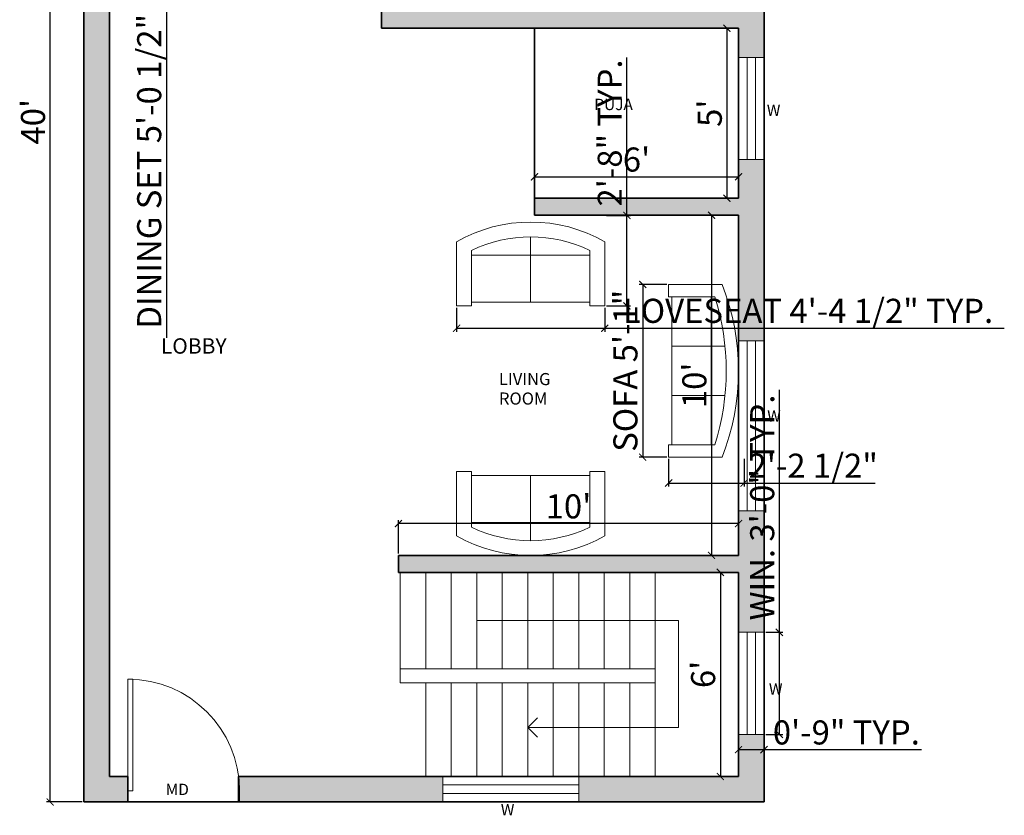
# Model space of a CAD drawing. Units: inches. Extents: x 3799 to 20199, y 1682 to 8087.
# Tile 28 of 30: x 17373 to 17720, y 7238 to 7519. Entities that reach past the tile are written whole.
import ezdxf

# ---------------------------------------------------------------- set-up
doc = ezdxf.new("R2010")
doc.units = ezdxf.units.IN
for name, color, linetype, lineweight in [('A-ANNO-DIMS', 2, 'Continuous', 18), ('A-ANNO-SYMB', 3, 'Continuous', 18), ('A-AREA-IDEN', 7, 'Continuous', 18), ('A-DOOR', 3, 'Continuous', 18), ('A-FLOR-STRS', 41, 'Continuous', 18), ('A-FURN', 8, 'Continuous', 18), ('A-GLAZ', 152, 'Continuous', 18), ('A-WALL', 7, 'Continuous', 35), ('A-WALL-PATT', 252, 'Continuous', 13)]:
    doc.layers.add(name, color=color, linetype=linetype, lineweight=lineweight)
doc.styles.get("Standard").update_dxf_attribs({"font": 'arial.ttf'})
doc.dimstyles.new('ISO-25', dxfattribs={"dimtxt": 8.5, "dimasz": 2.5, "dimexe": 1.25, "dimexo": 0.625, "dimtad": 1, "dimdec": 0, "dimlunit": 3, "dimtxsty": 'Standard', "dimblk": 'ARCHTICK', "dimcen": 2.5, "dimadec": 0, "dimazin": 0, "dimtfac": 1, "dimtdec": 0, "dimtmove": 0, "dimatfit": 3, "dimfxl": 1, "dimarcsym": 0})

# ---------------------------------------------------------------- blocks, each defined once
blk = doc.blocks.new('*U158')
for p, q in [((0, 0), (0, -100)), ((1000, 0), (1000, -100))]:
    blk.add_line(p, q)
blk.add_lwpolyline([(0, 0), (0, 1000), (43.75, 1000), (43.75, 0)], close=True)
blk.add_arc((0, 0), 1000, 0, 90)
blk = doc.blocks.new('Sofa - Roundback Loveseat 5 ft.')
for p, q in [((0, -32.44198), (0, -5.99998)), ((-24, -33.99998), (-24, -11.46958)), ((24.00004, -33.99998), (24.00004, -11.46958)), ((-23.9998, -13.38178), (23.99986, -13.38178)), ((-24, -32.44198), (24.00004, -32.44198))]:
    blk.add_line(p, q)
for points in [[(-24, -33.99998), (-30, -33.99998), (-30, -7.99998)], [(30.00004, -7.99998), (30.00004, -33.99998), (24.00004, -33.99998)]]:
    blk.add_lwpolyline(points)
for centre, radius, start, end in [((0, -60.24998), 60.24998, 60.13715, 119.8628), ((0, -61.38438), 55.38444, 64.32083, 115.6792)]:
    blk.add_arc(centre, radius, start, end)
blk = doc.blocks.new('Sofa - Roundback 7 ft.')
for p, q in [((-12.00002, -32.4421), (-12.00003, -6.5971)), ((11.99997, -32.4421), (11.99998, -6.5971)), ((-36.000027, -34), (-36.000027, -11.4696)), ((-35.999844, -13.3819), (35.9998, -13.3819)), ((35.99998, -34), (35.99998, -11.4696)), ((-36.000027, -32.4421), (35.99998, -32.4421))]:
    blk.add_line(p, q)
for points in [[(-36.000027, -34), (-42.000027, -34), (-42.000027, -8)], [(41.99998, -8), (41.99998, -34), (35.99998, -34)]]:
    blk.add_lwpolyline(points)
for centre, radius, start, end in [((0, -114.25), 114.25, 68.43141, 111.5686), ((-0.00001, -127.1968), 121.1968, 72.72033, 107.2797)]:
    blk.add_arc(centre, radius, start, end)
blk = doc.blocks.new('_ArchTick')
at = {"color": 0, "linetype": 'ByBlock', "const_width": 0.15}
blk.add_lwpolyline([(-0.5, -0.5), (0.5, 0.5)], dxfattribs=at)
blk = doc.blocks.new('*D163')
at = {"layer": 'A-ANNO-DIMS', "color": 0, "lineweight": -2, "transparency": 16777216}
for p, q in [((17554.17, 7456.64), (17554.17, 7464.85)), ((17554.17, 7463.6), (17626.17, 7463.6)), ((17626.17, 7456.64), (17626.17, 7464.85))]:
    blk.add_line(p, q, dxfattribs=at)
at = {"layer": 'Defpoints', "color": 0, "transparency": 16777216}
for p in [(17626.17, 7463.6), (17554.17, 7456.02), (17626.17, 7456.02)]:
    blk.add_point(p, dxfattribs=at)
at = {"layer": 'A-ANNO-DIMS', "color": 0, "lineweight": -2, "transparency": 16777216, "xscale": 2.5, "yscale": 2.5, "zscale": 2.5, "rotation": 180}
blk.add_blockref('_ArchTick', (17554.17, 7463.6), dxfattribs=at)
at = {"layer": 'A-ANNO-DIMS', "color": 0, "lineweight": -2, "transparency": 16777216, "xscale": 2.5, "yscale": 2.5, "zscale": 2.5}
blk.add_blockref('_ArchTick', (17626.17, 7463.6), dxfattribs=at)
at = {"layer": 'A-ANNO-DIMS', "color": 0, "transparency": 16777216, "insert": (17590.17, 7468.57), "char_height": 8.5, "attachment_point": 5}
blk.add_mtext("6'", dxfattribs=at)
blk = doc.blocks.new('*D164')
at = {"layer": 'A-ANNO-DIMS', "color": 0, "lineweight": -2, "transparency": 16777216}
for p, q in [((17625.55, 7516.02), (17620.81, 7516.02)), ((17622.06, 7516.02), (17622.06, 7456.02)), ((17625.55, 7456.02), (17620.81, 7456.02))]:
    blk.add_line(p, q, dxfattribs=at)
at = {"layer": 'Defpoints', "color": 0, "transparency": 16777216}
for p in [(17626.17, 7516.02), (17622.06, 7456.02), (17626.17, 7456.02)]:
    blk.add_point(p, dxfattribs=at)
at = {"layer": 'A-ANNO-DIMS', "color": 0, "lineweight": -2, "transparency": 16777216, "xscale": 2.5, "yscale": 2.5, "zscale": 2.5}
for p, rotation in [((17622.06, 7516.02), 90), ((17622.06, 7456.02), 270)]:
    blk.add_blockref('_ArchTick', p, dxfattribs=dict(at, rotation=rotation))
at = {"layer": 'A-ANNO-DIMS', "color": 0, "transparency": 16777216, "insert": (17617.11, 7486.02), "char_height": 8.5, "attachment_point": 5, "rotation": 90}
blk.add_mtext("5'", dxfattribs=at)
blk = doc.blocks.new('*D165')
at = {"layer": 'A-ANNO-DIMS', "color": 0, "lineweight": -2, "transparency": 16777216}
for p, q in [((17625.55, 7324.02), (17618.49, 7324.02)), ((17619.74, 7324.02), (17619.74, 7252.02)), ((17625.55, 7252.02), (17618.49, 7252.02))]:
    blk.add_line(p, q, dxfattribs=at)
at = {"layer": 'Defpoints', "color": 0, "transparency": 16777216}
for p in [(17626.17, 7324.02), (17619.74, 7252.02), (17626.17, 7252.02)]:
    blk.add_point(p, dxfattribs=at)
at = {"layer": 'A-ANNO-DIMS', "color": 0, "lineweight": -2, "transparency": 16777216, "xscale": 2.5, "yscale": 2.5, "zscale": 2.5}
for p, rotation in [((17619.74, 7324.02), 90), ((17619.74, 7252.02), 270)]:
    blk.add_blockref('_ArchTick', p, dxfattribs=dict(at, rotation=rotation))
at = {"layer": 'A-ANNO-DIMS', "color": 0, "transparency": 16777216, "insert": (17614.77, 7288.02), "char_height": 8.5, "attachment_point": 5, "rotation": 90}
blk.add_mtext("6'", dxfattribs=at)
blk = doc.blocks.new('*D166')
at = {"layer": 'A-ANNO-DIMS', "color": 0, "lineweight": -2, "transparency": 16777216}
for p, q in [((17625.55, 7450.02), (17615.39, 7450.02)), ((17616.64, 7450.02), (17616.64, 7330.02)), ((17625.55, 7330.02), (17615.39, 7330.02))]:
    blk.add_line(p, q, dxfattribs=at)
at = {"layer": 'Defpoints', "color": 0, "transparency": 16777216}
for p in [(17626.17, 7450.02), (17616.64, 7330.02), (17626.17, 7330.02)]:
    blk.add_point(p, dxfattribs=at)
at = {"layer": 'A-ANNO-DIMS', "color": 0, "lineweight": -2, "transparency": 16777216, "xscale": 2.5, "yscale": 2.5, "zscale": 2.5}
for p, rotation in [((17616.64, 7450.02), 90), ((17616.64, 7330.02), 270)]:
    blk.add_blockref('_ArchTick', p, dxfattribs=dict(at, rotation=rotation))
at = {"layer": 'A-ANNO-DIMS', "color": 0, "transparency": 16777216, "insert": (17611.68, 7390.02), "char_height": 8.5, "attachment_point": 5, "rotation": 90}
blk.add_mtext("10'", dxfattribs=at)
blk = doc.blocks.new('*D167')
at = {"layer": 'A-ANNO-DIMS', "color": 0, "lineweight": -2, "transparency": 16777216}
for p, q in [((17506.17, 7330.64), (17506.17, 7342.49)), ((17626.17, 7341.24), (17506.17, 7341.24)), ((17626.17, 7330.64), (17626.17, 7342.49))]:
    blk.add_line(p, q, dxfattribs=at)
at = {"layer": 'Defpoints', "color": 0, "transparency": 16777216}
for p in [(17506.17, 7341.24), (17506.17, 7330.02), (17626.17, 7330.02)]:
    blk.add_point(p, dxfattribs=at)
at = {"layer": 'A-ANNO-DIMS', "color": 0, "lineweight": -2, "transparency": 16777216, "xscale": 2.5, "yscale": 2.5, "zscale": 2.5, "rotation": 180}
blk.add_blockref('_ArchTick', (17506.17, 7341.24), dxfattribs=at)
at = {"layer": 'A-ANNO-DIMS', "color": 0, "lineweight": -2, "transparency": 16777216, "xscale": 2.5, "yscale": 2.5, "zscale": 2.5}
blk.add_blockref('_ArchTick', (17626.17, 7341.24), dxfattribs=at)
at = {"layer": 'A-ANNO-DIMS', "color": 0, "transparency": 16777216, "insert": (17566.17, 7346.21), "char_height": 8.5, "attachment_point": 5}
blk.add_mtext("10'", dxfattribs=at)
blk = doc.blocks.new('*D169')
at = {"layer": 'A-ANNO-DIMS', "color": 0, "lineweight": -2, "transparency": 16777216}
for p, q in [((17394.55, 7723.02), (17382.05, 7723.02)), ((17383.3, 7243.02), (17383.3, 7723.02)), ((17394.55, 7243.02), (17382.05, 7243.02))]:
    blk.add_line(p, q, dxfattribs=at)
at = {"layer": 'Defpoints', "color": 0, "transparency": 16777216}
for p in [(17383.3, 7723.02), (17395.17, 7723.02), (17395.17, 7243.02)]:
    blk.add_point(p, dxfattribs=at)
at = {"layer": 'A-ANNO-DIMS', "color": 0, "lineweight": -2, "transparency": 16777216, "xscale": 2.5, "yscale": 2.5, "zscale": 2.5}
for p, rotation in [((17383.3, 7723.02), 90), ((17383.3, 7243.02), 270)]:
    blk.add_blockref('_ArchTick', p, dxfattribs=dict(at, rotation=rotation))
at = {"layer": 'A-ANNO-DIMS', "color": 0, "transparency": 16777216, "insert": (17378.33, 7483.02), "char_height": 8.5, "attachment_point": 5, "rotation": 90}
blk.add_mtext("40'", dxfattribs=at)
blk = doc.blocks.new('WIN-48IN-9IN-FRAME')
for p, q in [((0, 0), (0, 9)), ((48, 0), (48, 9)), ((48, 6), (0, 6)), ((48, 3), (0, 3))]:
    blk.add_line(p, q)
blk = doc.blocks.new('WIN-60IN-9IN-FRAME')
for p, q in [((0, 9), (0, 0)), ((60, 9), (60, 0)), ((60, 6), (0, 6)), ((60, 3), (0, 3))]:
    blk.add_line(p, q)
blk = doc.blocks.new('WIN-36IN-9IN-FRAME')
for p, q in [((0, 36), (9, 36)), ((3, 36), (3, 0)), ((6, 36), (6, 0)), ((0, 0), (9, 0))]:
    blk.add_line(p, q)
blk = doc.blocks.new('*D264')
at = {"layer": 'A-ANNO-DIMS', "color": 0, "lineweight": -2, "transparency": 16777216}
for p, q in [((17600.88, 7425.63), (17591.11, 7425.63)), ((17592.36, 7425.63), (17592.36, 7364.67)), ((17600.88, 7364.67), (17591.11, 7364.67))]:
    blk.add_line(p, q, dxfattribs=at)
at = {"layer": 'Defpoints', "color": 0, "transparency": 16777216}
for p in [(17601.51, 7425.63), (17592.36, 7364.67), (17601.51, 7364.67)]:
    blk.add_point(p, dxfattribs=at)
at = {"layer": 'A-ANNO-DIMS', "color": 0, "lineweight": -2, "transparency": 16777216, "xscale": 2.5, "yscale": 2.5, "zscale": 2.5}
for p, rotation in [((17592.36, 7425.63), 90), ((17592.36, 7364.67), 270)]:
    blk.add_blockref('_ArchTick', p, dxfattribs=dict(at, rotation=rotation))
at = {"layer": 'A-ANNO-DIMS', "color": 0, "transparency": 16777216, "insert": (17587.34, 7395.15), "char_height": 8.5, "attachment_point": 5, "rotation": 90}
blk.add_mtext('SOFA 5\'-1"', dxfattribs=at)
blk = doc.blocks.new('*D265')
at = {"layer": 'A-ANNO-DIMS', "color": 0, "lineweight": -2, "transparency": 16777216}
for p, q in [((17601.51, 7364.05), (17601.51, 7354.28)), ((17628.11, 7364.05), (17628.11, 7354.28)), ((17601.51, 7355.53), (17628.11, 7355.53)), ((17628.11, 7355.53), (17674.41, 7355.53))]:
    blk.add_line(p, q, dxfattribs=at)
at = {"layer": 'Defpoints', "color": 0, "transparency": 16777216}
for p in [(17601.51, 7364.67), (17628.11, 7364.67), (17628.11, 7355.53)]:
    blk.add_point(p, dxfattribs=at)
at = {"layer": 'A-ANNO-DIMS', "color": 0, "lineweight": -2, "transparency": 16777216, "xscale": 2.5, "yscale": 2.5, "zscale": 2.5, "rotation": 180}
blk.add_blockref('_ArchTick', (17601.51, 7355.53), dxfattribs=at)
at = {"layer": 'A-ANNO-DIMS', "color": 0, "lineweight": -2, "transparency": 16777216, "xscale": 2.5, "yscale": 2.5, "zscale": 2.5}
blk.add_blockref('_ArchTick', (17628.11, 7355.53), dxfattribs=at)
at = {"layer": 'A-ANNO-DIMS', "color": 0, "transparency": 16777216, "insert": (17652.51, 7360.55), "char_height": 8.5, "attachment_point": 5}
blk.add_mtext('2\'-2 1/2"', dxfattribs=at)
blk = doc.blocks.new('*D280')
at = {"layer": 'A-ANNO-DIMS', "color": 0, "lineweight": -2, "transparency": 16777216}
for p, q in [((17526.69, 7417.39), (17526.69, 7408.92)), ((17578.95, 7417.39), (17578.95, 7408.92)), ((17526.69, 7410.17), (17578.95, 7410.17)), ((17578.95, 7410.17), (17719.93, 7410.17))]:
    blk.add_line(p, q, dxfattribs=at)
at = {"layer": 'Defpoints', "color": 0, "transparency": 16777216}
for p in [(17526.69, 7418.01), (17578.95, 7418.01), (17578.95, 7410.17)]:
    blk.add_point(p, dxfattribs=at)
at = {"layer": 'A-ANNO-DIMS', "color": 0, "lineweight": -2, "transparency": 16777216, "xscale": 2.5, "yscale": 2.5, "zscale": 2.5, "rotation": 180}
blk.add_blockref('_ArchTick', (17526.69, 7410.17), dxfattribs=at)
at = {"layer": 'A-ANNO-DIMS', "color": 0, "lineweight": -2, "transparency": 16777216, "xscale": 2.5, "yscale": 2.5, "zscale": 2.5}
blk.add_blockref('_ArchTick', (17578.95, 7410.17), dxfattribs=at)
at = {"layer": 'A-ANNO-DIMS', "color": 0, "transparency": 16777216, "insert": (17650.69, 7415.2), "char_height": 8.5, "attachment_point": 5}
blk.add_mtext('LOVESEAT 4\'-4 1/2" TYP.', dxfattribs=at)
blk = doc.blocks.new('*D281')
at = {"layer": 'A-ANNO-DIMS', "color": 0, "lineweight": -2, "transparency": 16777216}
for p, q in [((17586.78, 7449.95), (17586.78, 7505.65)), ((17579.57, 7449.95), (17588.03, 7449.95)), ((17586.78, 7418.01), (17586.78, 7449.95)), ((17579.57, 7418.01), (17588.03, 7418.01))]:
    blk.add_line(p, q, dxfattribs=at)
at = {"layer": 'Defpoints', "color": 0, "transparency": 16777216}
for p in [(17578.95, 7449.95), (17586.78, 7449.95), (17578.95, 7418.01)]:
    blk.add_point(p, dxfattribs=at)
at = {"layer": 'A-ANNO-DIMS', "color": 0, "lineweight": -2, "transparency": 16777216, "xscale": 2.5, "yscale": 2.5, "zscale": 2.5}
for p, rotation in [((17586.78, 7449.95), 90), ((17586.78, 7418.01), 270)]:
    blk.add_blockref('_ArchTick', p, dxfattribs=dict(at, rotation=rotation))
at = {"layer": 'A-ANNO-DIMS', "color": 0, "transparency": 16777216, "insert": (17581.82, 7479.05), "char_height": 8.5, "attachment_point": 5, "rotation": 90}
blk.add_mtext('2\'-8" TYP.', dxfattribs=at)
blk = doc.blocks.new('*D290')
at = {"layer": 'A-ANNO-DIMS', "color": 0, "lineweight": -2, "transparency": 16777216}
for p, q in [((17432.83, 7613.7), (17423.1, 7613.7)), ((17424.35, 7613.7), (17424.35, 7553.02)), ((17432.83, 7553.02), (17423.1, 7553.02)), ((17424.35, 7553.02), (17424.35, 7406.82))]:
    blk.add_line(p, q, dxfattribs=at)
at = {"layer": 'Defpoints', "color": 0, "transparency": 16777216}
for p in [(17433.46, 7613.7), (17424.35, 7553.02), (17433.46, 7553.02)]:
    blk.add_point(p, dxfattribs=at)
at = {"layer": 'A-ANNO-DIMS', "color": 0, "lineweight": -2, "transparency": 16777216, "xscale": 2.5, "yscale": 2.5, "zscale": 2.5}
for p, rotation in [((17424.35, 7613.7), 90), ((17424.35, 7553.02), 270)]:
    blk.add_blockref('_ArchTick', p, dxfattribs=dict(at, rotation=rotation))
at = {"layer": 'A-ANNO-DIMS', "color": 0, "transparency": 16777216, "insert": (17419.33, 7478.67), "char_height": 8.5, "attachment_point": 5, "rotation": 90}
blk.add_mtext('DINING SET 5\'-0 1/2" TYP.', dxfattribs=at)
blk = doc.blocks.new('*D338')
at = {"layer": 'A-ANNO-DIMS', "color": 0, "lineweight": -2, "transparency": 16777216}
for p, q in [((17640.57, 7302.87), (17640.57, 7388.46)), ((17635.8, 7302.87), (17641.82, 7302.87)), ((17640.57, 7266.87), (17640.57, 7302.87)), ((17635.8, 7266.87), (17641.82, 7266.87))]:
    blk.add_line(p, q, dxfattribs=at)
at = {"layer": 'Defpoints', "color": 0, "transparency": 16777216}
for p in [(17635.17, 7302.87), (17640.57, 7302.87), (17635.17, 7266.87)]:
    blk.add_point(p, dxfattribs=at)
at = {"layer": 'A-ANNO-DIMS', "color": 0, "lineweight": -2, "transparency": 16777216, "xscale": 2.5, "yscale": 2.5, "zscale": 2.5}
for p, rotation in [((17640.57, 7302.87), 90), ((17640.57, 7266.87), 270)]:
    blk.add_blockref('_ArchTick', p, dxfattribs=dict(at, rotation=rotation))
at = {"layer": 'A-ANNO-DIMS', "color": 0, "transparency": 16777216, "insert": (17635.61, 7346.92), "char_height": 8.5, "attachment_point": 5, "rotation": 90}
blk.add_mtext('WIN. 3\'-0" TYP.', dxfattribs=at)
blk = doc.blocks.new('*D339')
at = {"layer": 'A-ANNO-DIMS', "color": 0, "lineweight": -2, "transparency": 16777216}
for p, q in [((17626.17, 7266.25), (17626.17, 7260.22)), ((17635.17, 7266.25), (17635.17, 7260.22)), ((17626.17, 7261.47), (17635.17, 7261.47)), ((17635.17, 7261.47), (17690.73, 7261.47))]:
    blk.add_line(p, q, dxfattribs=at)
at = {"layer": 'Defpoints', "color": 0, "transparency": 16777216}
for p in [(17626.17, 7266.87), (17635.17, 7266.87), (17635.17, 7261.47)]:
    blk.add_point(p, dxfattribs=at)
at = {"layer": 'A-ANNO-DIMS', "color": 0, "lineweight": -2, "transparency": 16777216, "xscale": 2.5, "yscale": 2.5, "zscale": 2.5, "rotation": 180}
blk.add_blockref('_ArchTick', (17626.17, 7261.47), dxfattribs=at)
at = {"layer": 'A-ANNO-DIMS', "color": 0, "lineweight": -2, "transparency": 16777216, "xscale": 2.5, "yscale": 2.5, "zscale": 2.5}
blk.add_blockref('_ArchTick', (17635.17, 7261.47), dxfattribs=at)
at = {"layer": 'A-ANNO-DIMS', "color": 0, "transparency": 16777216, "insert": (17664.2, 7266.44), "char_height": 8.5, "attachment_point": 5}
blk.add_mtext('0\'-9" TYP.', dxfattribs=at)

msp = doc.modelspace()

# ---------------------------------------------------------------- hatches: boundary and pattern name
at = {"layer": 'A-WALL-PATT'}
h = msp.add_hatch(color=256, dxfattribs=at)
h.dxf.hatch_style = 1
h.paths.add_polyline_path([(17635.17, 7553.93), (17626.17, 7553.93), (17626.17, 7522.02), (17506.17, 7522.02), (17506.17, 7523.65), (17500.17, 7523.65), (17500.17, 7516.02), (17626.17, 7516.02), (17626.17, 7505.71), (17635.17, 7505.71)])
h.paths.add_polyline_path([(17404.17, 7550.08), (17395.17, 7550.08), (17395.17, 7243.02), (17410.75, 7243.02), (17410.75, 7252.02), (17404.17, 7252.02)])
h.paths.add_polyline_path([(17635.17, 7469.71), (17626.17, 7469.71), (17626.17, 7456.02), (17554.17, 7456.02), (17554.17, 7450.02), (17626.17, 7450.02), (17626.17, 7405.75), (17635.17, 7405.75)])
h.paths.add_polyline_path([(17635.17, 7345.75), (17626.17, 7345.75), (17626.17, 7330.02), (17555.18, 7330.02, -0.022507), (17550.46, 7330.02), (17506.17, 7330.02), (17506.17, 7324.02), (17626.17, 7324.02), (17626.17, 7302.87), (17635.17, 7302.87)])
h.paths.add_polyline_path([(17635.17, 7266.87), (17626.17, 7266.87), (17626.17, 7252.02), (17569.79, 7252.02), (17569.79, 7243.02), (17635.17, 7243.02)])
h.paths.add_polyline_path([(17521.79, 7252.02), (17449.79, 7252.02, -0.03225), (17450.12, 7246.96), (17450.12, 7243.02), (17521.79, 7243.02)])
h.paths.add_polyline_path([(17431.36, 7723.02), (17395.17, 7723.02), (17395.17, 7610.08), (17404.17, 7610.08), (17404.17, 7714.02), (17431.36, 7714.02)])
h.paths.add_polyline_path([(17635.17, 7723.02), (17479.36, 7723.02), (17479.36, 7714.02), (17500.17, 7714.02), (17500.17, 7559.65), (17506.17, 7559.65), (17506.17, 7636.02), (17511.5, 7636.02), (17511.5, 7642.02), (17506.17, 7642.02), (17506.17, 7714.02), (17626.17, 7714.02), (17626.17, 7691.04), (17635.17, 7691.04)])
h.paths.add_polyline_path([(17635.17, 7667.04), (17626.17, 7667.04), (17626.17, 7642.02), (17541.5, 7642.02), (17541.5, 7636.02), (17626.17, 7636.02), (17626.17, 7613.93), (17635.17, 7613.93)], flags=17)

# ---------------------------------------------------------------- linework, layer by layer
at = {"layer": 'A-FLOR-STRS'}
for p, q in [((17506.79, 7324.02), (17506.79, 7285.02)), ((17515.79, 7324.02), (17515.79, 7290.02)), ((17524.79, 7324.02), (17524.79, 7290.02)), ((17533.79, 7324.02), (17533.79, 7290.02)), ((17542.79, 7324.02), (17542.79, 7290.02)), ((17551.79, 7324.02), (17551.79, 7290.02)), ((17560.79, 7324.02), (17560.79, 7290.02)), ((17569.79, 7324.02), (17569.79, 7290.02)), ((17578.79, 7324.02), (17578.79, 7290.02)), ((17587.79, 7324.02), (17587.79, 7290.02)), ((17596.79, 7324.02), (17596.79, 7252.02)), ((17533.79, 7307.01), (17604.93, 7307.01)), ((17604.93, 7307.01), (17604.93, 7269.33)), ((17596.79, 7290.02), (17506.79, 7290.02)), ((17596.79, 7285.02), (17506.79, 7285.02)), ((17515.79, 7285.02), (17515.79, 7252.02)), ((17524.79, 7285.02), (17524.79, 7252.02)), ((17533.79, 7285.02), (17533.79, 7252.02)), ((17542.79, 7285.02), (17542.79, 7252.02)), ((17551.79, 7285.02), (17551.79, 7252.02)), ((17560.79, 7285.02), (17560.79, 7252.02)), ((17569.79, 7285.02), (17569.79, 7252.02)), ((17578.79, 7285.02), (17578.79, 7252.02)), ((17587.79, 7285.02), (17587.79, 7252.02)), ((17551.79, 7269.33), (17555.18, 7272.73)), ((17604.93, 7269.33), (17551.79, 7269.33)), ((17551.79, 7269.33), (17555.18, 7265.92))]:
    msp.add_line(p, q, dxfattribs=at)
at = {"layer": 'A-WALL'}
for p, q in [((17395.17, 7243.02), (17395.17, 7723.02)), ((17635.17, 7723.02), (17635.17, 7243.02)), ((17404.17, 7252.02), (17404.17, 7714.02)), ((17500.17, 7523.65), (17500.17, 7516.02)), ((17500.17, 7516.02), (17626.17, 7516.02)), ((17554.17, 7516.02), (17554.17, 7450.02)), ((17626.17, 7516.02), (17626.17, 7456.02)), ((17554.17, 7456.02), (17626.17, 7456.02)), ((17554.17, 7450.02), (17626.17, 7450.02)), ((17626.17, 7450.02), (17626.17, 7330.02)), ((17626.17, 7330.02), (17506.17, 7330.02)), ((17506.17, 7330.02), (17506.17, 7324.02)), ((17626.17, 7324.02), (17506.17, 7324.02)), ((17626.17, 7324.02), (17626.17, 7252.02)), ((17410.75, 7252.02), (17404.17, 7252.02)), ((17410.75, 7252.02), (17410.75, 7243.02)), ((17626.17, 7252.02), (17449.75, 7252.02)), ((17449.75, 7252.02), (17449.75, 7243.02)), ((17410.75, 7243.02), (17395.17, 7243.02)), ((17410.75, 7243.02), (17450.12, 7243.02)), ((17635.17, 7243.02), (17449.75, 7243.02))]:
    msp.add_line(p, q, dxfattribs=at)

# ---------------------------------------------------------------- block references
at = {"layer": 'A-DOOR', "xscale": 0.0393700787401575, "yscale": 0.0393700787401575, "zscale": 0.0393700787401575}
msp.add_blockref('*U158', (17410.75, 7246.96), dxfattribs=at)
at = {"layer": 'A-FURN', "xscale": 0.8709179497702034, "yscale": 0.8709179497702034, "zscale": 0.8709179497702034}
msp.add_blockref('Sofa - Roundback Loveseat 5 ft.', (17552.82, 7447.62), dxfattribs=at)
at = {"layer": 'A-FURN'}
for name, p, xscale, yscale, zscale, rotation in [('Sofa - Roundback 7 ft.', (17626.18, 7395.15), 0.7256888393464257, 0.7256888393464257, 0.7256888393464257, 270), ('Sofa - Roundback Loveseat 5 ft.', (17552.82, 7329.97), -0.8709179497702034, 0.8709179497702034, 0.8709179497702034, 180)]:
    msp.add_blockref(name, p, dxfattribs=dict(at, xscale=xscale, yscale=yscale, zscale=zscale, rotation=rotation))
at = {"layer": 'A-GLAZ'}
for name, p in [('WIN-36IN-9IN-FRAME', (17626.17, 7469.71)), ('WIN-36IN-9IN-FRAME', (17626.17, 7266.87)), ('WIN-48IN-9IN-FRAME', (17521.79, 7243.02))]:
    msp.add_blockref(name, p, dxfattribs=at)
at = {"layer": 'A-GLAZ', "rotation": 90}
msp.add_blockref('WIN-60IN-9IN-FRAME', (17635.17, 7345.75), dxfattribs=at)

# ---------------------------------------------------------------- texts
at = {"layer": 'A-ANNO-SYMB'}
for s, p in [('W', (17636.14, 7485.09)), ('W', (17636.27, 7377.24)), ('W', (17636.89, 7280.82)), ('MD', (17424.05, 7245.45)), ('W', (17542.29, 7238.3))]:
    msp.add_text(s, height=4, rotation=0.0011, dxfattribs=at).set_placement(p)
at = {"layer": 'A-AREA-IDEN'}
for s, height, p in [('PUJA', 4, (17575.25, 7487.12)), ('LOBBY', 5.436, (17422.33, 7401.18)), ('LIVING', 4.273, (17541.64, 7390.08)), ('ROOM', 4.273, (17541.64, 7383.21))]:
    msp.add_text(s, height=height, rotation=0.0011, dxfattribs=at).set_placement(p)

# ---------------------------------------------------------------- dimensions: what is measured, and where the dimension line sits
at = {"layer": 'A-ANNO-DIMS'}
for base, p1, p2, picture, middle in [((17383.3, 7723.02), (17395.17, 7243.02), (17395.17, 7723.02), '*D169', (17378.33, 7483.02)), ((17622.06, 7456.02), (17626.17, 7516.02), (17626.17, 7456.02), '*D164', (17617.11, 7486.02)), ((17616.64, 7330.02), (17626.17, 7450.02), (17626.17, 7330.02), '*D166', (17611.68, 7390.02)), ((17619.74, 7252.02), (17626.17, 7324.02), (17626.17, 7252.02), '*D165', (17614.77, 7288.02))]:
    dim = msp.add_linear_dim(base=base, p1=p1, p2=p2, angle=90, dimstyle='ISO-25', override={"dimclrd": 0, "dimclre": 0, "dimclrt": 0}, dxfattribs=at)
    dim.commit()
    dim.dimension.update_dxf_attribs({"geometry": picture, "text_midpoint": middle})
for base, p1, p2, angle, text, picture, middle in [((17424.35, 7553.02), (17433.46, 7613.7), (17433.46, 7553.02), 270, 'DINING SET <> TYP.', '*D290', (17419.33, 7478.67)), ((17586.78, 7449.95), (17578.95, 7418.01), (17578.95, 7449.95), 90, '<> TYP.', '*D281', (17581.82, 7479.05)), ((17592.36, 7364.67), (17601.51, 7425.63), (17601.51, 7364.67), 270, 'SOFA <>', '*D264', (17587.34, 7395.15)), ((17640.57, 7302.87), (17635.17, 7266.87), (17635.17, 7302.87), 90, 'WIN. <> TYP.', '*D338', (17635.61, 7346.92))]:
    dim = msp.add_linear_dim(base=base, p1=p1, p2=p2, angle=angle, text=text, dimstyle='ISO-25', override={"dimdec": 1, "dimlfac": 1, "dimrnd": 0, "dimzin": 1, "dimdsep": 46, "dimlunit": 4, "dimfrac": 2}, dxfattribs=at)
    dim.commit()
    dim.dimension.update_dxf_attribs({"geometry": picture, "text_midpoint": middle})
for base, p1, p2, override, picture, middle in [((17626.17, 7463.6), (17554.17, 7456.02), (17626.17, 7456.02), {"dimclrd": 0, "dimclre": 0, "dimclrt": 0}, '*D163', (17590.17, 7468.57)), ((17628.11, 7355.53), (17601.51, 7364.67), (17628.11, 7364.67), {"dimdec": 1, "dimlfac": 1, "dimrnd": 0, "dimzin": 1, "dimdsep": 46, "dimlunit": 4, "dimfrac": 2}, '*D265', (17652.51, 7360.55)), ((17506.17, 7341.24), (17626.17, 7330.02), (17506.17, 7330.02), {"dimclrd": 0, "dimclre": 0, "dimclrt": 0}, '*D167', (17566.17, 7346.21))]:
    dim = msp.add_linear_dim(base=base, p1=p1, p2=p2, dimstyle='ISO-25', override=override, dxfattribs=at)
    dim.commit()
    dim.dimension.update_dxf_attribs({"geometry": picture, "text_midpoint": middle})
for base, p1, p2, text, picture, middle in [((17578.95, 7410.17), (17526.69, 7418.01), (17578.95, 7418.01), 'LOVESEAT <> TYP.', '*D280', (17650.69, 7415.2)), ((17635.17, 7261.47), (17626.17, 7266.87), (17635.17, 7266.87), '<> TYP.', '*D339', (17664.2, 7266.44))]:
    dim = msp.add_linear_dim(base=base, p1=p1, p2=p2, text=text, dimstyle='ISO-25', override={"dimdec": 1, "dimlfac": 1, "dimrnd": 0, "dimzin": 1, "dimdsep": 46, "dimlunit": 4, "dimfrac": 2}, dxfattribs=at)
    dim.commit()
    dim.dimension.update_dxf_attribs({"geometry": picture, "text_midpoint": middle})

doc.saveas('drawing.dxf')
